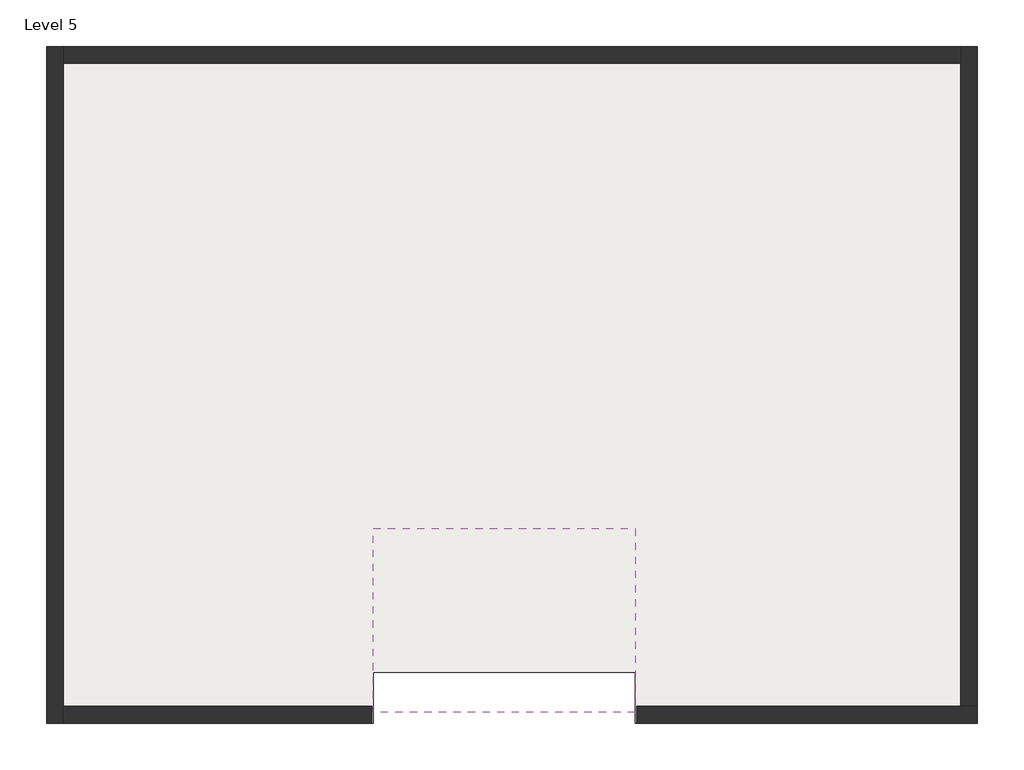
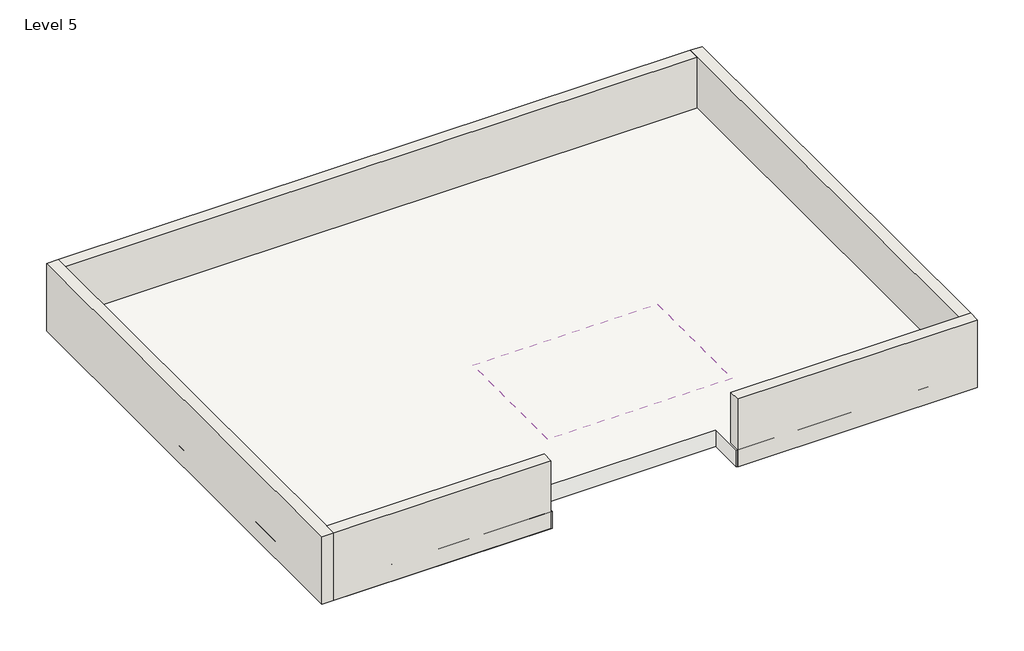
# One storey: 5 walls, 2 roofs.
"""IFC4 building model written with IfcOpenShell, lengths in millimetres."""

from ifc_helpers import new_model, si_unit, frame, origin, place, context, project, spatial, polyline, outline, extrude, faceted_brep, element, save

model = new_model("IFC4")

# Units and contexts
model_context = context("Model", 3, world=origin())
ifc_project = project(units=[si_unit("LENGTHUNIT", "METRE", prefix="MILLI")], contexts=[model_context])

# Site, building, storey
site = spatial("IfcSite", under=ifc_project)
building = spatial("IfcBuilding", under=site)
storey = spatial("IfcBuildingStorey", under=building, Name="Level 5", Elevation=14630.4)

# Roofs
placement = place(None, origin())
element("IfcRoof", 1, ObjectType="Generic - 12\"", at=placement, inside=storey, context=model_context, shape_type="SweptSolid", body=[
    extrude(outline(polyline([(-11016.1183714, 9432.6236997), (159.8816286, 9432.6236997), (159.8816286, 1304.6236997), (-3948.2087885, 1304.6236997), (-3948.2087885, 1914.2236997), (-7091.896639, 1914.2236997), (-7091.896639, 1304.6236997), (-11016.1183714, 1304.6236997), (-11016.1183714, 9432.6236997)])), frame((0.0, 0.0, 14630.4), z_axis=(0.0, 0.0, 1.0), x_axis=(1.0, 0.0, 0.0)), (0.0, 0.0, 1.0), 304.8),
])
element("IfcRoof", 2, ObjectType="Generic - 12\"", at=placement, inside=storey, context=model_context, shape_type="SweptSolid", body=[
    extrude(outline(polyline([(-7091.896639, 3641.4236997), (-3948.2087885, 3641.4236997), (-3948.2087885, 1431.6236997), (-7091.896639, 1431.6236997), (-7091.896639, 3641.4236997)])), frame((0.0, 0.0, 16154.4), z_axis=(0.0, 0.0, 1.0), x_axis=(1.0, 0.0, 0.0)), (0.0, 0.0, 1.0), 304.8),
])

# Walls
element("IfcWall", 3, ObjectType="Generic - 8\"", at=placement, inside=storey, context=model_context, shape_type="Brep", body=[
    faceted_brep([(-11016.1183714, 9432.6236997, 14630.4), (-11016.1183714, 1304.6236997, 14630.4), (-11016.1183714, 1304.6236997, 15849.6), (-11016.1183714, 9432.6236997, 15849.6), (-10812.9183714, 9432.6236997, 14630.4), (-10812.9183714, 9432.6236997, 15849.6), (-10812.9183714, 9229.4236997, 15849.6), (-10812.9183714, 1507.8236997, 15849.6), (-10812.9183714, 1304.6236997, 15849.6), (-10812.9183714, 1304.6236997, 14630.4), (-10812.9183714, 1507.8236997, 14630.4), (-10812.9183714, 9229.4236997, 14630.4)], [[[0, 1, 2, 3]], [[4, 5, 6, 7, 8, 9, 10, 11]], [[1, 0, 4, 11, 10, 9]], [[3, 2, 8, 7, 6, 5]], [[2, 1, 9, 8]], [[0, 3, 5, 4]]]),
])
element("IfcWall", 4, ObjectType="Generic - 8\"", at=placement, inside=storey, context=model_context, shape_type="SweptSolid", body=[
    extrude(outline(polyline([(-7110.8683714, 1304.6236997), (-10812.9183714, 1304.6236997), (-10812.9183714, 1507.8236997), (-7110.8683714, 1507.8236997), (-7110.8683714, 1304.6236997)])), frame((0.0, 0.0, 14630.4), z_axis=(0.0, 0.0, 1.0), x_axis=(1.0, 0.0, 0.0)), (0.0, 0.0, 1.0), 1219.2),
])
element("IfcWall", 5, ObjectType="Generic - 8\"", at=placement, inside=storey, context=model_context, shape_type="Brep", body=[
    faceted_brep([(-3929.5183714, 1304.6236997, 14630.4), (159.8816286, 1304.6236997, 14630.4), (159.8816286, 1304.6236997, 15849.6), (-3929.5183714, 1304.6236997, 15849.6), (-3929.5183714, 1507.8236997, 14630.4), (-3929.5183714, 1507.8236997, 15849.6), (-43.3183714, 1507.8236997, 15849.6), (159.8816286, 1507.8236997, 15849.6), (159.8816286, 1507.8236997, 14630.4), (-43.3183714, 1507.8236997, 14630.4)], [[[0, 1, 2, 3]], [[4, 5, 6, 7, 8, 9]], [[1, 0, 4, 9, 8]], [[3, 2, 7, 6, 5]], [[0, 3, 5, 4]], [[2, 1, 8, 7]]]),
])
element("IfcWall", 6, ObjectType="Generic - 8\"", at=placement, inside=storey, context=model_context, shape_type="Brep", body=[
    faceted_brep([(159.8816286, 1507.8236997, 14630.4), (159.8816286, 9432.6236997, 14630.4), (159.8816286, 9432.6236997, 15849.6), (159.8816286, 1507.8236997, 15849.6), (-43.3183714, 1507.8236997, 14630.4), (-43.3183714, 1507.8236997, 15849.6), (-43.3183714, 9229.4236997, 15849.6), (-43.3183714, 9432.6236997, 15849.6), (-43.3183714, 9432.6236997, 14630.4), (-43.3183714, 9229.4236997, 14630.4)], [[[0, 1, 2, 3]], [[4, 5, 6, 7, 8, 9]], [[1, 0, 4, 9, 8]], [[3, 2, 7, 6, 5]], [[0, 3, 5, 4]], [[2, 1, 8, 7]]]),
])
element("IfcWall", 7, ObjectType="Generic - 8\"", at=placement, inside=storey, context=model_context, shape_type="SweptSolid", body=[
    extrude(outline(polyline([(-10812.9183714, 9432.6236997), (-43.3183714, 9432.6236997), (-43.3183714, 9229.4236997), (-10812.9183714, 9229.4236997), (-10812.9183714, 9432.6236997)])), frame((0.0, 0.0, 14630.4), z_axis=(0.0, 0.0, 1.0), x_axis=(1.0, 0.0, 0.0)), (0.0, 0.0, 1.0), 1219.2),
])

save(model, "model.ifc")

# Revit data of these elements
# Type "Generic - 12\""
#   Assembly Code = "B1020"
#   Layers, outside or top first: 1' - 0" no material (function 1)
# Type "Generic - 8\""
#   Assembly Code = "B2010"
#   Layers, outside or top first: 0' - 8" no material (function 1)
# Element 1 (IfcRoof, "Generic - 12\"")
#   built-in parameter 1001705 = 49 (stored number, unit not read)
#   built-in parameter 1001710 = 33615
#   Phase Created = New Construction
#   Materials on its faces: "Default Roof"
# Element 2 (IfcRoof, "Generic - 12\"")
#   built-in parameter 1001705 = 54 (stored number, unit not read)
#   built-in parameter 1001701 = 5 (stored number, unit not read)
#   built-in parameter 1001710 = 33615
#   Phase Created = New Construction
#   Materials on its faces: "Default Roof"
# Elements 3, 4, 5, 6, 7 (IfcWall, "Generic - 8\"")
#   Top Offset = 0' - 0"
#   Base Offset = 0' - 0"
#   Unconnected Height = 4' - 0"
#   wall height = 4' - 0"
#   Phase Created = New Construction
#   Base Constraint = Level 5
#   Materials on its faces: "Default Wall"
# Materials
#   "Default Roof": colour RGB 88 101 114, transparency 0
#   "Default Wall": colour RGB 128 128 128, transparency 0
